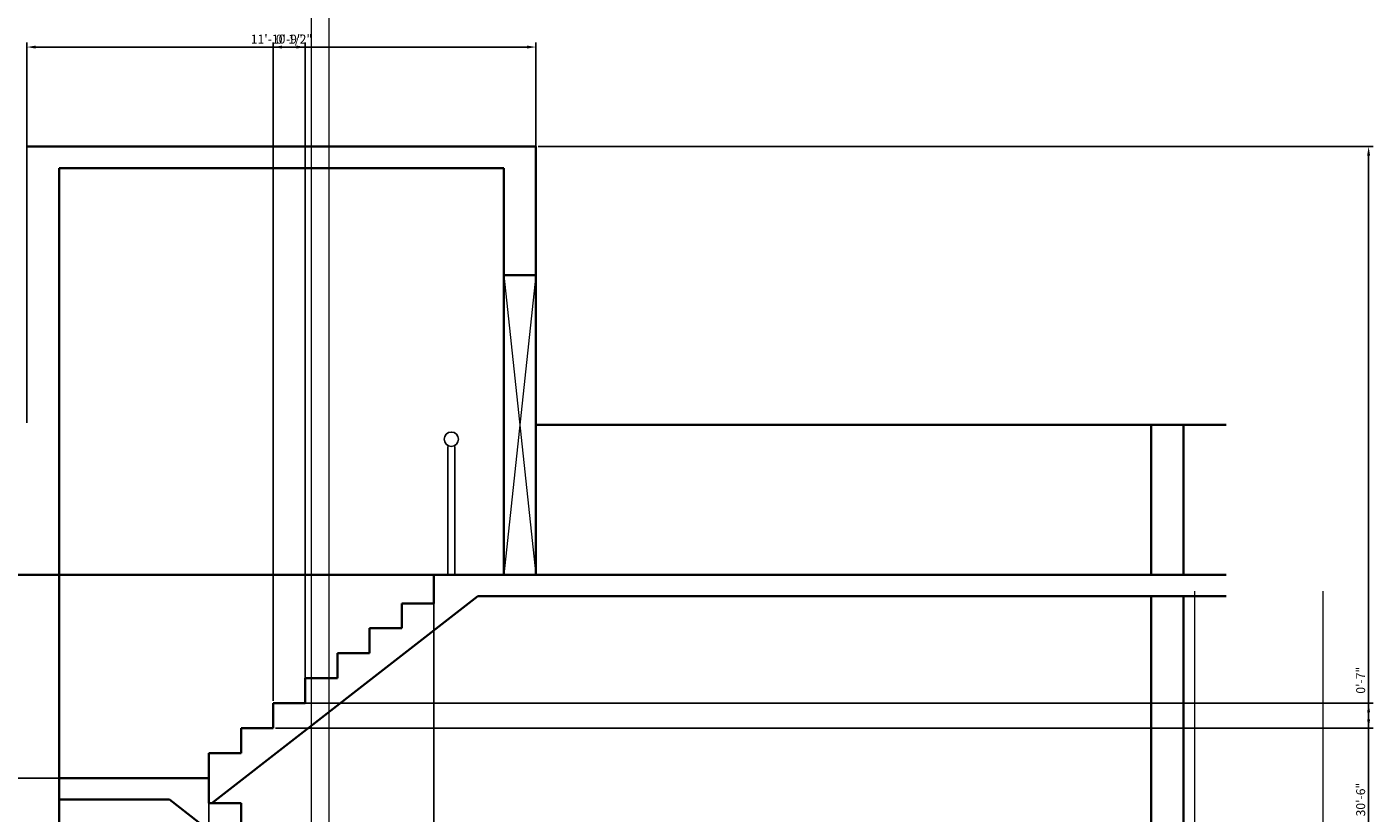
# Model space of a CAD drawing. Units: inches. Extents: x 2443635 to 2446153, y 1826255 to 1827341.
# Tile 14 of 16: x 2445143 to 2445520, y 1827042 to 1827262. Entities that reach past the tile are written whole.
import ezdxf

# ---------------------------------------------------------------- set-up
doc = ezdxf.new("R2010")
doc.units = ezdxf.units.IN
for name, color, linetype, lineweight in [('A-DIMS', 1, 'Continuous', 18), ('A-REFR', 8, 'Continuous', 13), ('A-SECT', 7, 'Continuous', 35), ('A-SECT-PROJ', 9, 'Continuous', 18), ('A-STAIR', 7, 'Continuous', 25)]:
    doc.layers.add(name, color=color, linetype=linetype, lineweight=lineweight)
doc.styles.get("Standard").update_dxf_attribs({"font": 'arial.ttf'})
doc.dimstyles.new('ISO-25', dxfattribs={"dimtxt": 2.5, "dimasz": 2.5, "dimexe": 1.25, "dimexo": 0.625, "dimtad": 1, "dimlunit": 4, "dimtxsty": 'Standard', "dimcen": 2.5, "dimadec": 0, "dimazin": 0, "dimtfac": 1, "dimtmove": 0, "dimatfit": 3, "dimfxl": 1, "dimarcsym": 0})

# ---------------------------------------------------------------- blocks, each defined once
blk = doc.blocks.new('*D99')
at = {"layer": 'A-DIMS', "color": 0, "lineweight": -2, "transparency": 16777216}
for p, q in [((2445286.12, 1827228.7), (2445520.01, 1827228.7)), ((2445518.76, 1826865.2), (2445518.76, 1827226.2)), ((2445143.49, 1826862.7), (2445520.01, 1826862.7))]:
    blk.add_line(p, q, dxfattribs=at)
at = {"layer": 'A-DIMS', "color": 0, "transparency": 16777216}
for points in [[(2445518.35, 1827226.2), (2445519.18, 1827226.2), (2445518.76, 1827228.7)], [(2445518.35, 1826865.2), (2445519.18, 1826865.2), (2445518.76, 1826862.7)]]:
    blk.add_solid(points, dxfattribs=at)
at = {"layer": 'Defpoints', "color": 0, "transparency": 16777216}
for p in [(2445285.49, 1827228.7), (2445518.76, 1827228.7), (2445142.86, 1826862.7)]:
    blk.add_point(p, dxfattribs=at)
at = {"layer": 'A-DIMS', "color": 0, "transparency": 16777216, "insert": (2445516.86, 1827045.7), "char_height": 2.5, "attachment_point": 5, "rotation": 90}
blk.add_mtext('30\'-6"', dxfattribs=at)
blk = doc.blocks.new('*D101')
at = {"layer": 'A-DIMS', "color": 0, "lineweight": -2, "transparency": 16777216}
for p, q in [((2445142.86, 1827151.33), (2445142.86, 1827257.85)), ((2445285.49, 1827151.33), (2445285.49, 1827257.85)), ((2445145.36, 1827256.6), (2445282.99, 1827256.6))]:
    blk.add_line(p, q, dxfattribs=at)
at = {"layer": 'A-DIMS', "color": 0, "transparency": 16777216}
for points in [[(2445145.36, 1827257.02), (2445145.36, 1827256.18), (2445142.86, 1827256.6)], [(2445282.99, 1827257.02), (2445282.99, 1827256.18), (2445285.49, 1827256.6)]]:
    blk.add_solid(points, dxfattribs=at)
at = {"layer": 'Defpoints', "color": 0, "transparency": 16777216}
for p in [(2445285.49, 1827256.6), (2445142.86, 1827150.7), (2445285.49, 1827150.7)]:
    blk.add_point(p, dxfattribs=at)
at = {"layer": 'A-DIMS', "color": 0, "transparency": 16777216, "insert": (2445214.18, 1827258.52), "char_height": 2.5, "attachment_point": 5}
blk.add_mtext('11\'-10 1/2"', dxfattribs=at)
blk = doc.blocks.new('*D102')
at = {"layer": 'A-DIMS', "color": 0, "lineweight": -2, "transparency": 16777216}
for p, q in [((2445151.86, 1827051.08), (2445151.86, 1826833.55)), ((2445193.86, 1827051.08), (2445193.86, 1826833.55)), ((2445154.36, 1826834.8), (2445191.36, 1826834.8))]:
    blk.add_line(p, q, dxfattribs=at)
at = {"layer": 'A-DIMS', "color": 0, "transparency": 16777216}
for points in [[(2445154.36, 1826835.22), (2445154.36, 1826834.38), (2445151.86, 1826834.8)], [(2445191.36, 1826835.22), (2445191.36, 1826834.38), (2445193.86, 1826834.8)]]:
    blk.add_solid(points, dxfattribs=at)
at = {"layer": 'Defpoints', "color": 0, "transparency": 16777216}
for p in [(2445151.86, 1827051.7), (2445193.86, 1827051.7), (2445193.86, 1826834.8)]:
    blk.add_point(p, dxfattribs=at)
at = {"layer": 'A-DIMS', "color": 0, "transparency": 16777216, "insert": (2445172.86, 1826836.7), "char_height": 2.5, "attachment_point": 5}
blk.add_mtext('3\'-6"', dxfattribs=at)
blk = doc.blocks.new('*D103')
at = {"layer": 'A-DIMS', "color": 0, "lineweight": -2, "transparency": 16777216}
for p, q in [((2445256.86, 1827108.08), (2445256.86, 1826833.55)), ((2445193.86, 1827051.08), (2445193.86, 1826833.55)), ((2445196.36, 1826834.8), (2445254.36, 1826834.8))]:
    blk.add_line(p, q, dxfattribs=at)
at = {"layer": 'A-DIMS', "color": 0, "transparency": 16777216}
for points in [[(2445196.36, 1826835.22), (2445196.36, 1826834.38), (2445193.86, 1826834.8)], [(2445254.36, 1826835.22), (2445254.36, 1826834.38), (2445256.86, 1826834.8)]]:
    blk.add_solid(points, dxfattribs=at)
at = {"layer": 'Defpoints', "color": 0, "transparency": 16777216}
for p in [(2445256.86, 1827108.7), (2445193.86, 1827051.7), (2445256.86, 1826834.8)]:
    blk.add_point(p, dxfattribs=at)
at = {"layer": 'A-DIMS', "color": 0, "transparency": 16777216, "insert": (2445225.36, 1826836.7), "char_height": 2.5, "attachment_point": 5}
blk.add_mtext('5\'-3"', dxfattribs=at)
blk = doc.blocks.new('*D104')
at = {"layer": 'A-DIMS', "color": 0, "lineweight": -2, "transparency": 16777216}
for p, q in [((2445256.24, 1827108.7), (2444992.25, 1827108.7)), ((2444993.5, 1827054.2), (2444993.5, 1827106.2)), ((2445193.24, 1827051.7), (2444992.25, 1827051.7))]:
    blk.add_line(p, q, dxfattribs=at)
at = {"layer": 'A-DIMS', "color": 0, "transparency": 16777216}
for points in [[(2444993.08, 1827106.2), (2444993.91, 1827106.2), (2444993.5, 1827108.7)], [(2444993.08, 1827054.2), (2444993.91, 1827054.2), (2444993.5, 1827051.7)]]:
    blk.add_solid(points, dxfattribs=at)
at = {"layer": 'Defpoints', "color": 0, "transparency": 16777216}
for p in [(2444993.5, 1827108.7), (2445256.86, 1827108.7), (2445193.86, 1827051.7)]:
    blk.add_point(p, dxfattribs=at)
at = {"layer": 'A-DIMS', "color": 0, "transparency": 16777216, "insert": (2444991.6, 1827080.2), "char_height": 2.5, "attachment_point": 5, "rotation": 90}
blk.add_mtext('4\'-9"', dxfattribs=at)
blk = doc.blocks.new('*D105')
at = {"layer": 'A-DIMS', "color": 0, "lineweight": -2, "transparency": 16777216}
for p, q in [((2445211.86, 1827073.33), (2445211.86, 1827257.85)), ((2445220.86, 1827073.33), (2445220.86, 1827257.85)), ((2445214.36, 1827256.6), (2445218.36, 1827256.6))]:
    blk.add_line(p, q, dxfattribs=at)
at = {"layer": 'A-DIMS', "color": 0, "transparency": 16777216}
for points in [[(2445214.36, 1827257.02), (2445214.36, 1827256.18), (2445211.86, 1827256.6)], [(2445218.36, 1827257.02), (2445218.36, 1827256.18), (2445220.86, 1827256.6)]]:
    blk.add_solid(points, dxfattribs=at)
at = {"layer": 'Defpoints', "color": 0, "transparency": 16777216}
for p in [(2445220.86, 1827256.6), (2445211.86, 1827072.7), (2445220.86, 1827072.7)]:
    blk.add_point(p, dxfattribs=at)
at = {"layer": 'A-DIMS', "color": 0, "transparency": 16777216, "insert": (2445216.36, 1827258.5), "char_height": 2.5, "attachment_point": 5}
blk.add_mtext('0\'-9"', dxfattribs=at)
blk = doc.blocks.new('*D106')
at = {"layer": 'A-DIMS', "color": 0, "lineweight": -2, "transparency": 16777216}
for p, q in [((2445518.76, 1827072.7), (2445518.76, 1827083.1)), ((2445212.49, 1827072.7), (2445520.01, 1827072.7)), ((2445518.76, 1827068.2), (2445518.76, 1827070.2)), ((2445212.49, 1827065.7), (2445520.01, 1827065.7))]:
    blk.add_line(p, q, dxfattribs=at)
at = {"layer": 'A-DIMS', "color": 0, "transparency": 16777216}
for points in [[(2445518.35, 1827070.2), (2445519.18, 1827070.2), (2445518.76, 1827072.7)], [(2445518.35, 1827068.2), (2445519.18, 1827068.2), (2445518.76, 1827065.7)]]:
    blk.add_solid(points, dxfattribs=at)
at = {"layer": 'Defpoints', "color": 0, "transparency": 16777216}
for p in [(2445211.86, 1827072.7), (2445518.76, 1827072.7), (2445211.86, 1827065.7)]:
    blk.add_point(p, dxfattribs=at)
at = {"layer": 'A-DIMS', "color": 0, "transparency": 16777216, "insert": (2445516.86, 1827079.15), "char_height": 2.5, "attachment_point": 5, "rotation": 90}
blk.add_mtext('0\'-7"', dxfattribs=at)

msp = doc.modelspace()

# ---------------------------------------------------------------- linework, layer by layer
at = {"layer": 'A-REFR'}
for p, q in [((2445469.966, 1827104.133), (2445469.966, 1826329.288)), ((2445505.966, 1827104.133), (2445505.966, 1826329.288))]:
    msp.add_line(p, q, dxfattribs=at)
at = {"layer": 'A-REFR', "transparency": 33554687}
for p in [(2445227.466, 1827321.207), (2445222.466, 1827316.303)]:
    msp.add_ray(p, (0, -1), dxfattribs=at)
at = {"layer": 'A-SECT'}
for p, q in [((2445285.491, 1827228.701), (2445142.864, 1827228.701)), ((2445285.491, 1827228.701), (2445285.491, 1827108.701)), ((2445151.864, 1827222.701), (2445151.864, 1826868.701)), ((2445276.491, 1827222.701), (2445151.864, 1827222.701)), ((2445276.491, 1827222.701), (2445276.491, 1827108.701)), ((2445285.491, 1827192.701), (2445276.491, 1827192.701)), ((2445478.864, 1827150.701), (2445285.491, 1827150.701)), ((2445457.864, 1827150.701), (2445457.864, 1827108.701)), ((2445466.864, 1827150.701), (2445466.864, 1827108.701)), ((2445478.864, 1827108.701), (2445021.398, 1827108.701)), ((2445256.864, 1827108.701), (2445256.864, 1827100.701)), ((2445194.637, 1827044.701), (2445269.208, 1827102.701)), ((2445256.864, 1827100.701), (2445247.864, 1827100.701)), ((2445247.864, 1827100.701), (2445247.864, 1827093.701)), ((2445478.864, 1827102.701), (2445269.208, 1827102.701)), ((2445457.864, 1827102.701), (2445457.864, 1826988.701)), ((2445466.864, 1827102.701), (2445466.864, 1826982.701)), ((2445247.864, 1827093.701), (2445238.864, 1827093.701)), ((2445238.864, 1827093.701), (2445238.864, 1827086.701)), ((2445238.864, 1827086.701), (2445229.864, 1827086.701)), ((2445229.864, 1827086.701), (2445229.864, 1827079.701)), ((2445229.864, 1827079.701), (2445220.864, 1827079.701)), ((2445220.864, 1827079.701), (2445220.864, 1827072.701)), ((2445220.864, 1827072.701), (2445211.864, 1827072.701)), ((2445211.864, 1827072.701), (2445211.864, 1827065.701)), ((2445211.864, 1827065.701), (2445202.864, 1827065.701)), ((2445202.864, 1827065.701), (2445202.864, 1827058.701)), ((2445202.864, 1827058.701), (2445193.864, 1827058.701)), ((2445193.864, 1827058.701), (2445193.864, 1827051.701)), ((2445193.864, 1827051.701), (2445151.864, 1827051.701)), ((2445193.864, 1827051.701), (2445151.864, 1827051.701)), ((2445193.864, 1827044.701), (2445193.864, 1827051.701)), ((2445182.805, 1827045.701), (2445151.864, 1827045.701)), ((2445256.864, 1826988.1), (2445182.805, 1827045.701)), ((2445202.864, 1827044.701), (2445193.864, 1827044.701)), ((2445202.864, 1827037.701), (2445202.864, 1827044.701))]:
    msp.add_line(p, q, dxfattribs=at)
at = {"layer": 'A-SECT-PROJ'}
for p, q in [((2445285.491, 1827192.701), (2445276.491, 1827108.701)), ((2445276.491, 1827192.701), (2445285.491, 1827108.701))]:
    msp.add_line(p, q, dxfattribs=at)
at = {"layer": 'A-STAIR'}
for p, q in [((2445260.765, 1827108.701), (2445260.765, 1827144.701)), ((2445262.765, 1827108.701), (2445262.765, 1827144.701))]:
    msp.add_line(p, q, dxfattribs=at)
msp.add_circle((2445261.767, 1827146.701), 2, dxfattribs=at)

# ---------------------------------------------------------------- dimensions: what is measured, and where the dimension line sits
at = {"layer": 'A-DIMS', "transparency": 33554687}
for base, p1, p2, picture, middle in [((2445285.491, 1827256.601), (2445142.864, 1827150.701), (2445285.491, 1827150.701), '*D101', (2445214.177, 1827258.519)), ((2445220.864, 1827256.601), (2445211.864, 1827072.701), (2445220.864, 1827072.701), '*D105', (2445216.364, 1827258.503)), ((2445256.864, 1826834.801), (2445193.864, 1827051.701), (2445256.864, 1827108.701), '*D103', (2445225.364, 1826836.703)), ((2445193.864, 1826834.801), (2445151.864, 1827051.701), (2445193.864, 1827051.701), '*D102', (2445172.864, 1826836.703))]:
    dim = msp.add_linear_dim(base=base, p1=p1, p2=p2, dimstyle='ISO-25', override={"dimdec": 1, "dimlfac": 1, "dimrnd": 0, "dimzin": 1, "dimdsep": 46, "dimlunit": 4, "dimfrac": 2}, dxfattribs=at)
    dim.commit()
    dim.dimension.update_dxf_attribs({"geometry": picture, "text_midpoint": middle})
for base, p1, p2, picture, middle in [((2445518.764, 1827228.701), (2445142.864, 1826862.701), (2445285.491, 1827228.701), '*D99', (2445516.861, 1827045.701)), ((2444993.498, 1827108.701), (2445193.864, 1827051.701), (2445256.864, 1827108.701), '*D104', (2444991.596, 1827080.201)), ((2445518.764, 1827072.701), (2445211.864, 1827065.701), (2445211.864, 1827072.701), '*D106', (2445516.862, 1827079.149))]:
    dim = msp.add_linear_dim(base=base, p1=p1, p2=p2, angle=90, dimstyle='ISO-25', override={"dimdec": 1, "dimlfac": 1, "dimrnd": 0, "dimzin": 1, "dimdsep": 46, "dimlunit": 4, "dimfrac": 2}, dxfattribs=at)
    dim.commit()
    dim.dimension.update_dxf_attribs({"geometry": picture, "text_midpoint": middle})

doc.saveas('drawing.dxf')
